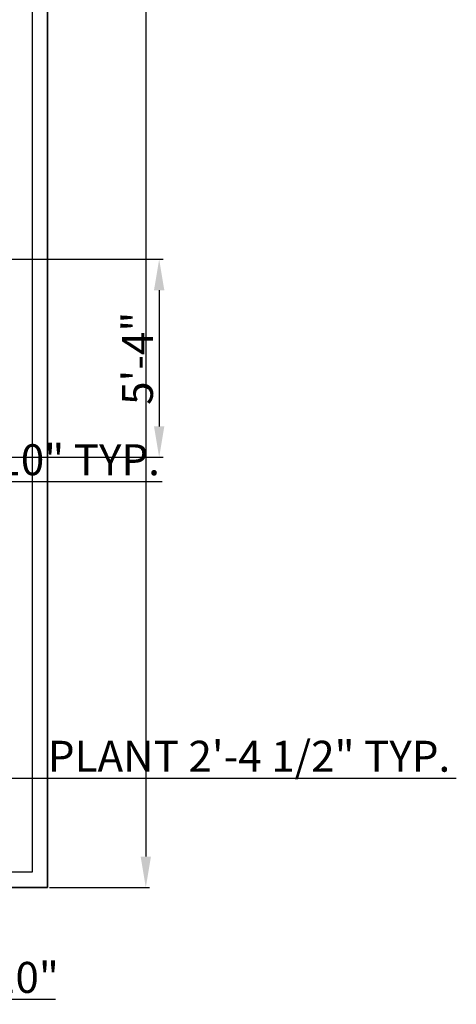
# Model space of a CAD drawing. Units: inches. Extents: x 2206 to 2843, y 1750 to 2489.
# Tile 4 of 8: x 2702 to 2843, y 1757 to 2075. Entities that reach past the tile are written whole.
import ezdxf

# ---------------------------------------------------------------- set-up
doc = ezdxf.new("R2010")
doc.units = ezdxf.units.IN
for name, color, linetype, lineweight in [('A-ANNO-DIMS', 2, 'Continuous', 18), ('C-PROP', 7, 'Continuous', 35), ('L-SITE-WALL', 8, 'Continuous', 25)]:
    doc.layers.add(name, color=color, linetype=linetype, lineweight=lineweight)
doc.styles.get("Standard").update_dxf_attribs({"font": 'arial.ttf'})
doc.dimstyles.new('ISO-25', dxfattribs={"dimtxt": 10, "dimasz": 10, "dimexe": 1.25, "dimexo": 0.625, "dimtad": 1, "dimdec": 1, "dimlunit": 3, "dimtxsty": 'Standard', "dimcen": 2.5, "dimadec": 0, "dimazin": 0, "dimtfac": 1, "dimtdec": 1, "dimtmove": 0, "dimatfit": 3, "dimfxl": 1, "dimarcsym": 0})

# ---------------------------------------------------------------- blocks, each defined once
blk = doc.blocks.new('*D15')
at = {"layer": 'A-ANNO-DIMS', "color": 0, "lineweight": -2, "transparency": 16777216}
for p, q in [((2711.2, 2394.9), (2743.56, 2394.9)), ((2742.31, 2384.9), (2742.31, 1804.9)), ((2711.2, 1794.9), (2743.56, 1794.9))]:
    blk.add_line(p, q, dxfattribs=at)
at = {"layer": 'A-ANNO-DIMS', "color": 0, "transparency": 16777216}
for points in [[(2740.65, 2384.9), (2743.98, 2384.9), (2742.31, 2394.9)], [(2740.65, 1804.9), (2743.98, 1804.9), (2742.31, 1794.9)]]:
    blk.add_solid(points, dxfattribs=at)
at = {"layer": 'Defpoints', "color": 0, "transparency": 16777216}
for p in [(2710.58, 2394.9), (2710.58, 1794.9), (2742.31, 1794.9)]:
    blk.add_point(p, dxfattribs=at)
at = {"layer": 'A-ANNO-DIMS', "color": 0, "transparency": 16777216, "insert": (2736.58, 2094.9), "char_height": 10, "attachment_point": 5, "rotation": 90}
blk.add_mtext("50'", dxfattribs=at)
blk = doc.blocks.new('*D27')
at = {"layer": 'A-ANNO-DIMS', "color": 0, "lineweight": -2, "transparency": 16777216}
for p, q in [((2670.31, 1826.6), (2670.31, 1831.49)), ((2680.31, 1830.24), (2688.72, 1830.24)), ((2698.72, 1826.6), (2698.72, 1831.49)), ((2698.72, 1830.24), (2842.63, 1830.24))]:
    blk.add_line(p, q, dxfattribs=at)
at = {"layer": 'A-ANNO-DIMS', "color": 0, "transparency": 16777216}
for points in [[(2680.31, 1831.91), (2680.31, 1828.57), (2670.31, 1830.24)], [(2688.72, 1831.91), (2688.72, 1828.57), (2698.72, 1830.24)]]:
    blk.add_solid(points, dxfattribs=at)
at = {"layer": 'Defpoints', "color": 0, "transparency": 16777216}
for p in [(2698.72, 1830.24), (2670.31, 1825.98), (2698.72, 1825.98)]:
    blk.add_point(p, dxfattribs=at)
at = {"layer": 'A-ANNO-DIMS', "color": 0, "transparency": 16777216, "insert": (2775.67, 1836.03), "char_height": 10, "attachment_point": 5}
blk.add_mtext('PLANT 2\'-4 1/2" TYP.', dxfattribs=at)
blk = doc.blocks.new('*D40')
at = {"layer": 'A-ANNO-DIMS', "color": 0, "lineweight": -2, "transparency": 16777216}
for p, q in [((2637.58, 1926.1), (2627.58, 1926.1)), ((2647.58, 1919.52), (2647.58, 1927.35)), ((2647.58, 1926.1), (2657.58, 1926.1)), ((2657.58, 1919.52), (2657.58, 1927.35)), ((2667.58, 1926.1), (2747.55, 1926.1))]:
    blk.add_line(p, q, dxfattribs=at)
at = {"layer": 'A-ANNO-DIMS', "color": 0, "transparency": 16777216}
for points in [[(2637.58, 1927.77), (2637.58, 1924.43), (2647.58, 1926.1)], [(2667.58, 1927.77), (2667.58, 1924.43), (2657.58, 1926.1)]]:
    blk.add_solid(points, dxfattribs=at)
at = {"layer": 'Defpoints', "color": 0, "transparency": 16777216}
for p in [(2657.58, 1926.1), (2647.58, 1918.9), (2657.58, 1918.9)]:
    blk.add_point(p, dxfattribs=at)
at = {"layer": 'A-ANNO-DIMS', "color": 0, "transparency": 16777216, "insert": (2712.57, 1931.83), "char_height": 10, "attachment_point": 5}
blk.add_mtext('0\'-10" TYP.', dxfattribs=at)
blk = doc.blocks.new('*D63')
at = {"layer": 'A-ANNO-DIMS', "color": 0, "lineweight": -2, "transparency": 16777216}
for p, q in [((2647.58, 2246.27), (2647.58, 1757.6)), ((2657.58, 2246.27), (2657.58, 1757.6)), ((2637.58, 1758.85), (2627.58, 1758.85)), ((2647.58, 1758.85), (2657.58, 1758.85)), ((2667.58, 1758.85), (2713.18, 1758.85))]:
    blk.add_line(p, q, dxfattribs=at)
at = {"layer": 'A-ANNO-DIMS', "color": 0, "transparency": 16777216}
for points in [[(2637.58, 1760.52), (2637.58, 1757.18), (2647.58, 1758.85)], [(2667.58, 1760.52), (2667.58, 1757.18), (2657.58, 1758.85)]]:
    blk.add_solid(points, dxfattribs=at)
at = {"layer": 'Defpoints', "color": 0, "transparency": 16777216}
for p in [(2647.58, 2246.9), (2657.58, 2246.9), (2657.58, 1758.85)]:
    blk.add_point(p, dxfattribs=at)
at = {"layer": 'A-ANNO-DIMS', "color": 0, "transparency": 16777216, "insert": (2695.38, 1764.58), "char_height": 10, "attachment_point": 5}
blk.add_mtext('0\'-10"', dxfattribs=at)
blk = doc.blocks.new('*D69')
at = {"layer": 'A-ANNO-DIMS', "color": 0, "lineweight": -2, "transparency": 16777216}
for p, q in [((2658.2, 1997.9), (2747.88, 1997.9)), ((2746.63, 1987.9), (2746.63, 1943.9)), ((2648.2, 1933.9), (2747.88, 1933.9))]:
    blk.add_line(p, q, dxfattribs=at)
at = {"layer": 'A-ANNO-DIMS', "color": 0, "transparency": 16777216}
for points in [[(2744.96, 1987.9), (2748.3, 1987.9), (2746.63, 1997.9)], [(2744.96, 1943.9), (2748.3, 1943.9), (2746.63, 1933.9)]]:
    blk.add_solid(points, dxfattribs=at)
at = {"layer": 'Defpoints', "color": 0, "transparency": 16777216}
for p in [(2657.58, 1997.9), (2647.58, 1933.9), (2746.63, 1933.9)]:
    blk.add_point(p, dxfattribs=at)
at = {"layer": 'A-ANNO-DIMS', "color": 0, "transparency": 16777216, "insert": (2740.92, 1965.9), "char_height": 10, "attachment_point": 5, "rotation": 90}
blk.add_mtext('5\'-4"', dxfattribs=at)

msp = doc.modelspace()

# ---------------------------------------------------------------- linework, layer by layer
at = {"layer": 'C-PROP'}
for p, q in [((2710.58, 2394.9), (2710.58, 1794.9)), ((2710.58, 1794.9), (2254.58, 1794.9))]:
    msp.add_line(p, q, dxfattribs=at)
at = {"layer": 'L-SITE-WALL'}
for p, q in [((2705.58, 2290.9), (2705.58, 1799.9)), ((2705.58, 1799.9), (2259.58, 1799.9))]:
    msp.add_line(p, q, dxfattribs=at)

# ---------------------------------------------------------------- dimensions: what is measured, and where the dimension line sits
at = {"layer": 'A-ANNO-DIMS'}
for base, p1, p2, override, picture, middle in [((2742.31, 1794.9), (2710.58, 2394.9), (2710.58, 1794.9), {"dimclrd": 0, "dimclre": 0, "dimclrt": 0}, '*D15', (2736.58, 2094.9)), ((2746.63, 1933.9), (2657.58, 1997.9), (2647.58, 1933.9), {"dimdec": 1, "dimlfac": 1, "dimrnd": 0, "dimzin": 1, "dimdsep": 46, "dimlunit": 4, "dimfrac": 2}, '*D69', (2740.92, 1965.9))]:
    dim = msp.add_linear_dim(base=base, p1=p1, p2=p2, angle=90, dimstyle='ISO-25', override=override, dxfattribs=at)
    dim.commit()
    dim.dimension.update_dxf_attribs({"geometry": picture, "text_midpoint": middle})
dim = msp.add_linear_dim(base=(2657.58, 1758.85), p1=(2647.58, 2246.9), p2=(2657.58, 2246.9), dimstyle='ISO-25', override={"dimdec": 1, "dimlfac": 1, "dimrnd": 0, "dimzin": 1, "dimdsep": 46, "dimlunit": 4, "dimfrac": 2}, dxfattribs=at)
dim.commit()
dim.dimension.update_dxf_attribs({"geometry": '*D63', "text_midpoint": (2695.38, 1764.58)})
for base, p1, p2, text, picture, middle in [((2657.58, 1926.1), (2647.58, 1918.9), (2657.58, 1918.9), '<> TYP.', '*D40', (2712.57, 1931.83)), ((2698.72, 1830.24), (2670.31, 1825.98), (2698.72, 1825.98), 'PLANT <> TYP.', '*D27', (2775.67, 1836.03))]:
    dim = msp.add_linear_dim(base=base, p1=p1, p2=p2, text=text, dimstyle='ISO-25', override={"dimdec": 1, "dimlfac": 1, "dimrnd": 0, "dimzin": 1, "dimdsep": 46, "dimlunit": 4, "dimfrac": 2}, dxfattribs=at)
    dim.commit()
    dim.dimension.update_dxf_attribs({"geometry": picture, "text_midpoint": middle})

doc.saveas('drawing.dxf')
